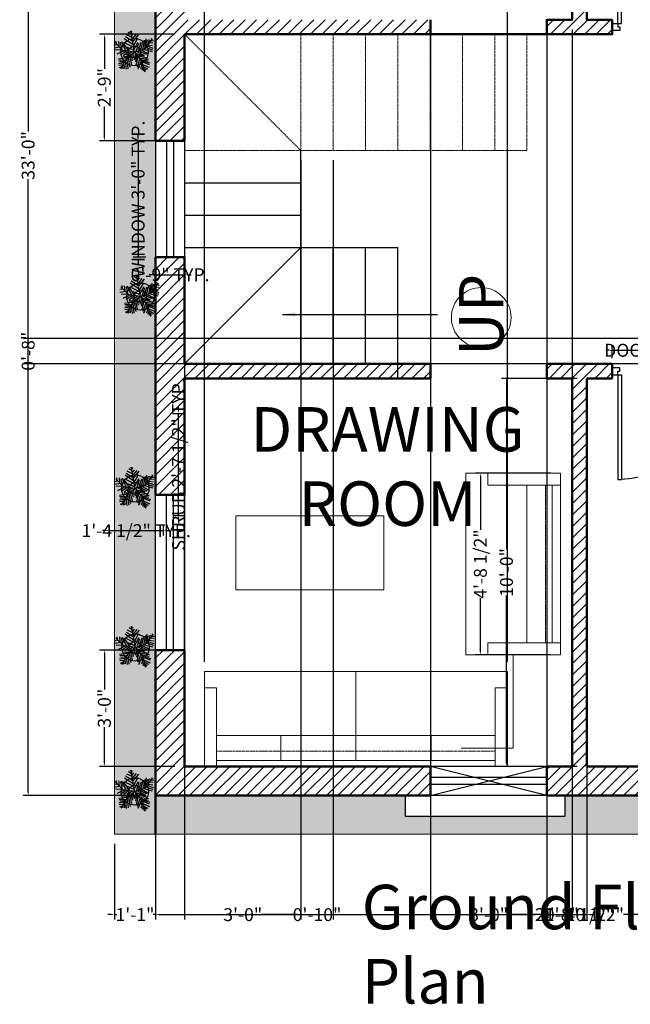
# Model space of a CAD drawing. Units: inches. Extents: x 1265938 to 1266301, y 2357745 to 2358240.
# Tile 1 of 4: x 1265942 to 1266131, y 2357745 to 2358050. Entities that reach past the tile are written whole.
import ezdxf

# ---------------------------------------------------------------- set-up
doc = ezdxf.new("R2010")
doc.units = ezdxf.units.IN
doc.header["$MEASUREMENT"] = 0
doc.linetypes.add('20230926_Unit Plans$0$HIDDEN', pattern=[0.375, 0.25, -0.125])
for name, color, linetype, lineweight in [('A-ANNO-SYMB', 7, 'Continuous', 18), ('A-ANNO-TEXT', 7, 'Continuous', 25), ('A-AREA-IDEN', 7, 'Continuous', 18), ('A-DOOR', 4, 'Continuous', 25), ('A-FLOR-STRS', 7, 'Continuous', 25), ('A-FLOR-STRS-OVHD', 6, '20230926_Unit Plans$0$HIDDEN', 18), ('A-FURN', 8, 'Continuous', 18), ('A-FURN-HIDN', 8, '20230926_Unit Plans$0$HIDDEN', 13), ('A-WALL-PATT', 8, 'Continuous', 13), ('L-PLNT', 3, 'Continuous', 18), ('L-PLNT-BEDS', 3, 'Continuous', 18), ('L-PLNT-PATT', 3, 'Continuous', 13), ('WALL', 7, 'Continuous', 50), ('WINDOW', 2, 'Continuous', 25), ('YQ_DIM', 3, 'Continuous', 18)]:
    doc.layers.add(name, color=color, linetype=linetype, lineweight=lineweight)
doc.layers.add('Layer2', color=102, linetype='Continuous')
doc.layers.add('RAMP SLOPE', color=8, linetype='Continuous')
doc.styles.get("Standard").update_dxf_attribs({"font": 'arial.ttf'})
doc.styles.add('YQ_DIM', font='SUPEROS.SHX', dxfattribs={"width": 0.8, "bigfont": 'HZDX.SHX'})
doc.dimstyles.new('yqi0', dxfattribs={"dimscale": 0, "dimtxt": 4, "dimasz": 1, "dimexe": 1.5, "dimexo": 3, "dimgap": 0.5, "dimtad": 0, "dimdsep": 46, "dimlunit": 4, "dimtxsty": 'Standard', "dimcen": 0, "dimclrd": 256, "dimclre": 256, "dimclrt": 7, "dimadec": 1, "dimazin": 2, "dimtfac": 1, "dimtix": 1, "dimtmove": 2, "dimatfit": 2, "dimfxl": 1, "dimtolj": 1, "dimtzin": 0, "dimarcsym": 0})

# ---------------------------------------------------------------- blocks, each defined once
blk = doc.blocks.new('WD_WIN4')
for p, q in [((-0.5, 0.5), (0.5, 0.5)), ((-0.5, 0.12), (0.5, 0.12)), ((-0.5, -0.12), (0.5, -0.12)), ((-0.5, -0.5), (0.5, -0.5))]:
    blk.add_line(p, q)
blk = doc.blocks.new('DR_D01')
for p, q in [((-0.45, 0.93), (-0.42, 0.93)), ((-0.45, 0.03), (-0.45, 0.93)), ((-0.42, 0.03), (-0.42, 0.93)), ((-0.5, 0.03), (-0.42, 0.03)), ((-0.5, 0.03), (-0.5, -0.03)), ((-0.45, 0.03), (-0.45, 0)), ((-0.45, 0), (-0.435, 0)), ((-0.435, 0), (-0.435, -0.03)), ((0.435, 0), (0.435, -0.03)), ((0.45, 0), (0.435, 0)), ((0.45, 0.03), (0.45, 0)), ((0.5, 0.03), (0.45, 0.03)), ((0.5, -0.03), (0.5, 0.03)), ((-0.435, -0.03), (-0.5, -0.03)), ((0.435, -0.03), (0.5, -0.03))]:
    blk.add_line(p, q)
blk.add_arc((-0.4602, 0.0206), 0.9103, 0.59152, 87.46644)
blk = doc.blocks.new('Trees - Metric')
at = {"layer": 'Layer2'}
for p, q in [((-258.7244, 1362.456), (-332.3336, 1421.4348)), ((0, 0), (-266.7, 1447.8)), ((-231.1146, 1315.2628), (-166.7002, 1421.4348)), ((-1234.059, 536.7274), (-1252.4486, 737.2604)), ((-1105.2302, 725.4494), (-1077.6458, 395.1732)), ((-902.8176, 713.6638), (-617.5756, 100.2538)), ((-93.091, 489.5342), (-700.3796, 902.3858)), ((-129.8956, 713.6638), (-626.7704, 1032.1544)), ((-185.1152, 1008.5578), (-553.1612, 1185.4942)), ((-221.9198, 1197.3052), (-433.5526, 1338.8594)), ((-194.31, 1102.9442), (-65.4812, 1256.284)), ((-148.3106, 914.1968), (118.5418, 1220.9018)), ((-129.8956, 701.8528), (265.7602, 1185.4942)), ((-74.7014, 418.7444), (219.7608, 961.39)), ((-28.6766, 171.0436), (228.9556, 678.2816)), ((412.9786, 147.447), (587.8068, 796.2392)), ((560.197, 182.8292), (698.2206, 819.8358)), ((685.8, 228.6), (1219.2, 914.4)), ((689.0258, 230.0224), (790.2448, 914.1968)), ((808.6344, 784.4282), (827.0494, 418.7444)), ((891.4384, 831.6214), (946.658, 572.1096)), ((983.4626, 867.0036), (1066.2666, 725.4494)), ((1112.2914, 760.8316), (1296.3144, 784.4282)), ((1121.4862, 925.9824), (1149.0706, 831.6214)), ((-1206.4492, 501.3198), (-1418.082, 465.9376)), ((-1031.621, 347.98), (-1399.667, 277.1902)), ((-800.1, 114.3), (-1333.5, 647.7)), ((-847.598, 159.2326), (-1326.0578, 135.636)), ((-718.7946, 88.4682), (-1215.644, -147.447)), ((-976.4268, 666.4706), (-884.4026, 194.6402)), ((-543.9664, 76.6572), (-967.2066, -206.4512)), ((0, 0), (-800.1, 114.3)), ((-369.1382, 53.086), (-783.1836, 642.874)), ((-405.9428, 53.086), (-764.794, -241.8334)), ((-617.5756, 607.4918), (-74.7014, 347.98)), ((0, 0), (-571.5, -495.3)), ((-166.7002, 29.4894), (-543.9664, -206.4512)), ((-525.5514, 347.98), (-28.6766, 123.8504)), ((0, 0), (685.8, 228.6)), ((0, 0), (457.2, -571.5)), ((100.1268, 41.275), (284.1498, 619.2774)), ((164.5412, 41.275), (661.416, -218.2368)), ((256.5654, 88.4682), (449.7832, 666.4706)), ((284.1498, 88.4682), (781.0246, -147.447)), ((458.978, 147.447), (891.4384, -88.4682)), ((615.4166, 194.6402), (1185.8752, 41.275)), ((753.4148, 312.5978), (1222.6798, 159.2326)), ((845.439, 418.7444), (1241.0948, 277.1902)), ((919.0482, 501.3198), (1222.6798, 454.152)), ((1029.462, 654.685), (1241.0948, 631.0884)), ((-442.7474, -383.3876), (-1086.8406, -477.7486)), ((-617.5756, -548.5384), (-1077.6458, -560.324)), ((-681.9646, -666.496), (-1022.4262, -654.685)), ((-571.5, -495.3), (-952.5, -1143)), ((-387.5278, -324.4088), (-764.794, -324.4088)), ((-635.9652, -607.5172), (-580.771, -1150.1374)), ((-525.5514, -465.963), (-451.9422, -1126.5408)), ((-166.7002, -147.447), (-507.1618, -253.619)), ((-433.5526, -383.3876), (-323.1134, -1020.3688)), ((-341.5284, -289.0012), (-221.9198, -831.6214)), ((-240.3094, -218.2368), (-157.5054, -595.7062)), ((-120.7008, -88.4682), (-93.091, -371.5766)), ((63.3222, -76.6826), (-37.8714, -513.1308)), ((44.9326, -64.897), (615.4166, -241.8334)), ((127.7366, -159.258), (54.1274, -654.685)), ((228.9556, -289.0012), (90.932, -914.1968)), ((357.759, -430.5554), (164.5412, -1020.3688)), ((192.151, -230.0224), (817.8292, -371.5766)), ((458.978, -572.1096), (210.5406, -1161.923)), ((311.7596, -383.3876), (937.4378, -477.7486)), ((412.9786, -501.3452), (919.0482, -583.9206)), ((457.2, -571.5), (685.8, -1333.5)), ((468.1982, -572.1096), (1029.462, -737.2604)), ((486.5878, -642.8994), (983.4626, -843.4324)), ((-718.7946, -737.2604), (-1086.8406, -796.2392)), ((-783.1836, -867.029), (-1077.6458, -902.4112)), ((-875.2078, -1008.5832), (-1040.8412, -1079.3476)), ((-829.2084, -937.7934), (-810.7934, -1126.5408)), ((-737.1842, -784.4536), (-709.5744, -1114.7298)), ((514.1976, -772.6426), (403.7838, -1138.3264)), ((578.612, -961.39), (495.7826, -1232.7128)), ((541.8074, -831.6214), (992.6574, -1032.1544)), ((578.612, -973.1756), (873.0488, -1138.3264)), ((624.6114, -1161.923), (587.8068, -1291.6916)), ((624.6114, -1102.9442), (781.0246, -1209.1162)), ((679.8056, -1268.095), (716.6102, -1291.6916))]:
    blk.add_line(p, q, dxfattribs=at)
blk = doc.blocks.new('A$Cbdbf8f2b')
at = {"layer": 'RAMP SLOPE'}
for radius in [7.17, 3.22]:
    blk.add_circle((13.77, 14.11), radius, dxfattribs=at)
at = {"xscale": 0.0077264756515533, "yscale": 0.0077264756515533, "zscale": 0.0077264756515533}
blk.add_blockref('Trees - Metric', (13.77, 14.11), dxfattribs=at)
blk = doc.blocks.new('*D16')
at = {"layer": 'Defpoints', "color": 0, "transparency": 16777216}
for p in [(1265986.27, 2357927.89), (1265991, 2357927.89), (1265986.27, 2357896.34)]:
    blk.add_point(p, dxfattribs=at)
at = {"layer": 'YQ_DIM', "lineweight": -2, "transparency": 16777216}
for p, q in [((1265991, 2357928.89), (1265991, 2357929.89)), ((1265989.27, 2357927.89), (1265992.5, 2357927.89)), ((1265991, 2357896.34), (1265991, 2357927.89)), ((1265989.27, 2357896.34), (1265992.5, 2357896.34)), ((1265991, 2357895.34), (1265991, 2357894.34))]:
    blk.add_line(p, q, dxfattribs=at)
at = {"layer": 'YQ_DIM', "transparency": 16777216}
for points in [[(1265990.83, 2357928.89), (1265991.16, 2357928.89), (1265991, 2357927.89)], [(1265990.83, 2357895.34), (1265991.16, 2357895.34), (1265991, 2357896.34)]]:
    blk.add_solid(points, dxfattribs=at)
at = {"layer": 'YQ_DIM', "color": 7, "transparency": 16777216, "insert": (1265991, 2357912.11), "char_height": 4, "attachment_point": 5, "rotation": 90}
blk.add_mtext('\\A1;SHRUB 2\'-7 1/2" TYP.', dxfattribs=at)
blk = doc.blocks.new('*D17')
at = {"layer": 'Defpoints', "color": 0, "transparency": 16777216}
for p in [(1265969.52, 2357896.34), (1265986.27, 2357896.34), (1265986.27, 2357891.61)]:
    blk.add_point(p, dxfattribs=at)
at = {"layer": 'YQ_DIM', "lineweight": -2, "transparency": 16777216}
for p, q in [((1265969.52, 2357893.34), (1265969.52, 2357890.11)), ((1265986.27, 2357893.34), (1265986.27, 2357890.11)), ((1265968.52, 2357891.61), (1265967.52, 2357891.61)), ((1265969.52, 2357891.61), (1265986.27, 2357891.61)), ((1265987.27, 2357891.61), (1265988.27, 2357891.61))]:
    blk.add_line(p, q, dxfattribs=at)
at = {"layer": 'YQ_DIM', "transparency": 16777216}
for points in [[(1265968.52, 2357891.78), (1265968.52, 2357891.44), (1265969.52, 2357891.61)], [(1265987.27, 2357891.78), (1265987.27, 2357891.44), (1265986.27, 2357891.61)]]:
    blk.add_solid(points, dxfattribs=at)
at = {"layer": 'YQ_DIM', "color": 7, "transparency": 16777216, "insert": (1265977.89, 2357891.61), "char_height": 4, "attachment_point": 5}
blk.add_mtext('\\A1;1\'-4 1/2" TYP.', dxfattribs=at)
blk = doc.blocks.new('*D22')
at = {"layer": 'Defpoints', "color": 0, "transparency": 16777216}
for p in [(1265983.89, 2358012.18), (1265978.49, 2357976.18), (1265983.89, 2357976.18)]:
    blk.add_point(p, dxfattribs=at)
at = {"layer": 'YQ_DIM', "lineweight": -2, "transparency": 16777216}
for p, q in [((1265978.49, 2358013.18), (1265978.49, 2358014.18)), ((1265980.89, 2358012.18), (1265976.99, 2358012.18)), ((1265978.49, 2358012.18), (1265978.49, 2357976.18)), ((1265980.89, 2357976.18), (1265976.99, 2357976.18)), ((1265978.49, 2357975.18), (1265978.49, 2357974.18))]:
    blk.add_line(p, q, dxfattribs=at)
at = {"layer": 'YQ_DIM', "transparency": 16777216}
for points in [[(1265978.32, 2358013.18), (1265978.66, 2358013.18), (1265978.49, 2358012.18)], [(1265978.32, 2357975.18), (1265978.66, 2357975.18), (1265978.49, 2357976.18)]]:
    blk.add_solid(points, dxfattribs=at)
at = {"layer": 'YQ_DIM', "color": 7, "transparency": 16777216, "insert": (1265978.49, 2357994.18), "char_height": 4, "attachment_point": 5, "rotation": 90}
blk.add_mtext('\\A1;WINDOW 3\'-0" TYP.', dxfattribs=at)
blk = doc.blocks.new('*D23')
at = {"layer": 'Defpoints', "color": 0, "transparency": 16777216}
for p in [(1265983.89, 2357976.18), (1265992.89, 2357976.18), (1265992.89, 2357970.78)]:
    blk.add_point(p, dxfattribs=at)
at = {"layer": 'YQ_DIM', "lineweight": -2, "transparency": 16777216}
for p, q in [((1265983.89, 2357973.18), (1265983.89, 2357969.28)), ((1265992.89, 2357973.18), (1265992.89, 2357969.28)), ((1265982.89, 2357970.78), (1265981.89, 2357970.78)), ((1265983.89, 2357970.78), (1265992.89, 2357970.78)), ((1265993.89, 2357970.78), (1265994.89, 2357970.78))]:
    blk.add_line(p, q, dxfattribs=at)
at = {"layer": 'YQ_DIM', "transparency": 16777216}
for points in [[(1265982.89, 2357970.95), (1265982.89, 2357970.61), (1265983.89, 2357970.78)], [(1265993.89, 2357970.95), (1265993.89, 2357970.61), (1265992.89, 2357970.78)]]:
    blk.add_solid(points, dxfattribs=at)
at = {"layer": 'YQ_DIM', "color": 7, "transparency": 16777216, "insert": (1265988.39, 2357970.78), "char_height": 4, "attachment_point": 5}
blk.add_mtext('\\A1;0\'-9" TYP.', dxfattribs=at)
blk = doc.blocks.new('*D26')
at = {"layer": 'Defpoints', "color": 0, "transparency": 16777216}
for p in [(1266161.26, 2357947.41), (1266125.26, 2357942.01), (1266161.26, 2357942.01)]:
    blk.add_point(p, dxfattribs=at)
at = {"layer": 'YQ_DIM', "lineweight": -2, "transparency": 16777216}
for p, q in [((1266124.26, 2357947.41), (1266123.26, 2357947.41)), ((1266125.26, 2357945.01), (1266125.26, 2357948.91)), ((1266125.26, 2357947.41), (1266161.26, 2357947.41)), ((1266161.26, 2357945.01), (1266161.26, 2357948.91)), ((1266162.26, 2357947.41), (1266163.26, 2357947.41))]:
    blk.add_line(p, q, dxfattribs=at)
at = {"layer": 'YQ_DIM', "transparency": 16777216}
for points in [[(1266124.26, 2357947.58), (1266124.26, 2357947.24), (1266125.26, 2357947.41)], [(1266162.26, 2357947.58), (1266162.26, 2357947.24), (1266161.26, 2357947.41)]]:
    blk.add_solid(points, dxfattribs=at)
at = {"layer": 'YQ_DIM', "color": 7, "transparency": 16777216, "insert": (1266143.26, 2357947.41), "char_height": 4, "attachment_point": 5}
blk.add_mtext('\\A1;DOOR 3\'-0" TYP.', dxfattribs=at)
blk = doc.blocks.new('*D36')
at = {"layer": 'Defpoints', "color": 0, "transparency": 16777216}
for p in [(1265983.89, 2357809.68), (1266246.39, 2357809.68), (1266246.39, 2357772.83)]:
    blk.add_point(p, dxfattribs=at)
at = {"layer": 'YQ_DIM', "lineweight": -2, "transparency": 16777216}
for p, q in [((1265983.89, 2357806.68), (1265983.89, 2357771.33)), ((1266246.39, 2357806.68), (1266246.39, 2357771.33)), ((1265984.89, 2357772.83), (1266101.52, 2357772.83)), ((1266245.39, 2357772.83), (1266128.76, 2357772.83))]:
    blk.add_line(p, q, dxfattribs=at)
at = {"layer": 'YQ_DIM', "transparency": 16777216}
for points in [[(1265984.89, 2357773), (1265984.89, 2357772.66), (1265983.89, 2357772.83)], [(1266245.39, 2357773), (1266245.39, 2357772.66), (1266246.39, 2357772.83)]]:
    blk.add_solid(points, dxfattribs=at)
at = {"layer": 'YQ_DIM', "color": 7, "transparency": 16777216, "insert": (1266115.14, 2357772.83), "char_height": 4, "attachment_point": 5}
blk.add_mtext('\\A1;21\'-10 1/2"', dxfattribs=at)
blk = doc.blocks.new('*D37')
at = {"layer": 'Defpoints', "color": 0, "transparency": 16777216}
for p in [(1265944.45, 2358205.68), (1265983.89, 2358205.68), (1265983.89, 2357809.68)]:
    blk.add_point(p, dxfattribs=at)
at = {"layer": 'YQ_DIM', "lineweight": -2, "transparency": 16777216}
for p, q in [((1265980.89, 2358205.68), (1265942.95, 2358205.68)), ((1265944.45, 2358204.68), (1265944.45, 2358015.05)), ((1265944.45, 2357810.68), (1265944.45, 2358000.31)), ((1265980.89, 2357809.68), (1265942.95, 2357809.68))]:
    blk.add_line(p, q, dxfattribs=at)
at = {"layer": 'YQ_DIM', "transparency": 16777216}
for points in [[(1265944.29, 2358204.68), (1265944.62, 2358204.68), (1265944.45, 2358205.68)], [(1265944.29, 2357810.68), (1265944.62, 2357810.68), (1265944.45, 2357809.68)]]:
    blk.add_solid(points, dxfattribs=at)
at = {"layer": 'YQ_DIM', "color": 7, "transparency": 16777216, "insert": (1265944.45, 2358007.68), "char_height": 4, "attachment_point": 5, "rotation": 90}
blk.add_mtext('\\A1;33\'-0"', dxfattribs=at)
blk = doc.blocks.new('*D42')
at = {"layer": 'Defpoints', "color": 0, "transparency": 16777216}
for p in [(1266092.54, 2357938.68), (1266117.39, 2357938.68), (1266117.39, 2357818.68)]:
    blk.add_point(p, dxfattribs=at)
at = {"layer": 'YQ_DIM', "lineweight": -2, "transparency": 16777216}
for p, q in [((1266114.39, 2357938.68), (1266091.04, 2357938.68)), ((1266092.54, 2357937.68), (1266092.54, 2357885.86)), ((1266092.54, 2357819.68), (1266092.54, 2357871.5)), ((1266114.39, 2357818.68), (1266091.04, 2357818.68))]:
    blk.add_line(p, q, dxfattribs=at)
at = {"layer": 'YQ_DIM', "transparency": 16777216}
for points in [[(1266092.37, 2357937.68), (1266092.71, 2357937.68), (1266092.54, 2357938.68)], [(1266092.37, 2357819.68), (1266092.71, 2357819.68), (1266092.54, 2357818.68)]]:
    blk.add_solid(points, dxfattribs=at)
at = {"layer": 'YQ_DIM', "color": 7, "transparency": 16777216, "insert": (1266092.54, 2357878.68), "char_height": 4, "attachment_point": 5, "rotation": 90}
blk.add_mtext('\\A1;10\'-0"', dxfattribs=at)
blk = doc.blocks.new('*D43')
at = {"layer": 'Defpoints', "color": 0, "transparency": 16777216}
for p in [(1265968.04, 2357854.68), (1265992.89, 2357854.68), (1265992.89, 2357818.68)]:
    blk.add_point(p, dxfattribs=at)
at = {"layer": 'YQ_DIM', "lineweight": -2, "transparency": 16777216}
for p, q in [((1265989.89, 2357854.68), (1265966.54, 2357854.68)), ((1265968.04, 2357853.68), (1265968.04, 2357842.5)), ((1265968.04, 2357819.68), (1265968.04, 2357830.87)), ((1265989.89, 2357818.68), (1265966.54, 2357818.68))]:
    blk.add_line(p, q, dxfattribs=at)
at = {"layer": 'YQ_DIM', "transparency": 16777216}
for points in [[(1265967.87, 2357853.68), (1265968.21, 2357853.68), (1265968.04, 2357854.68)], [(1265967.87, 2357819.68), (1265968.21, 2357819.68), (1265968.04, 2357818.68)]]:
    blk.add_solid(points, dxfattribs=at)
at = {"layer": 'YQ_DIM', "color": 7, "transparency": 16777216, "insert": (1265968.04, 2357836.68), "char_height": 4, "attachment_point": 5, "rotation": 90}
blk.add_mtext('\\A1;3\'-0"', dxfattribs=at)
blk = doc.blocks.new('*D44')
at = {"layer": 'Defpoints', "color": 0, "transparency": 16777216}
for p in [(1265968.04, 2358045.18), (1265992.89, 2358045.18), (1265992.89, 2358012.18)]:
    blk.add_point(p, dxfattribs=at)
at = {"layer": 'YQ_DIM', "lineweight": -2, "transparency": 16777216}
for p, q in [((1265989.89, 2358045.18), (1265966.54, 2358045.18)), ((1265968.04, 2358044.18), (1265968.04, 2358034.53)), ((1265968.04, 2358013.18), (1265968.04, 2358022.83)), ((1265989.89, 2358012.18), (1265966.54, 2358012.18))]:
    blk.add_line(p, q, dxfattribs=at)
at = {"layer": 'YQ_DIM', "transparency": 16777216}
for points in [[(1265967.87, 2358044.18), (1265968.21, 2358044.18), (1265968.04, 2358045.18)], [(1265967.87, 2358013.18), (1265968.21, 2358013.18), (1265968.04, 2358012.18)]]:
    blk.add_solid(points, dxfattribs=at)
at = {"layer": 'YQ_DIM', "color": 7, "transparency": 16777216, "insert": (1265968.04, 2358028.68), "char_height": 4, "attachment_point": 5, "rotation": 90}
blk.add_mtext('\\A1;2\'-9"', dxfattribs=at)
blk = doc.blocks.new('*D48')
at = {"layer": 'Defpoints', "color": 0, "transparency": 16777216}
for p in [(1266105.02, 2357818.68), (1266112.89, 2357818.68), (1266112.89, 2357772.83)]:
    blk.add_point(p, dxfattribs=at)
at = {"layer": 'YQ_DIM', "lineweight": -2, "transparency": 16777216}
for p, q in [((1266105.02, 2357815.68), (1266105.02, 2357771.33)), ((1266112.89, 2357815.68), (1266112.89, 2357771.33)), ((1266104.02, 2357772.83), (1266103.02, 2357772.83)), ((1266105.02, 2357772.83), (1266112.89, 2357772.83)), ((1266113.89, 2357772.83), (1266114.89, 2357772.83))]:
    blk.add_line(p, q, dxfattribs=at)
at = {"layer": 'YQ_DIM', "transparency": 16777216}
for points in [[(1266104.02, 2357773), (1266104.02, 2357772.66), (1266105.02, 2357772.83)], [(1266113.89, 2357773), (1266113.89, 2357772.66), (1266112.89, 2357772.83)]]:
    blk.add_solid(points, dxfattribs=at)
at = {"layer": 'YQ_DIM', "color": 7, "transparency": 16777216, "insert": (1266108.96, 2357772.83), "char_height": 4, "attachment_point": 5}
blk.add_mtext('\\A1;0\'-8"', dxfattribs=at)
blk = doc.blocks.new('*D49')
at = {"layer": 'Defpoints', "color": 0, "transparency": 16777216}
for p in [(1266125.26, 2358237.77), (1266117.39, 2358049.68), (1266125.26, 2358049.68)]:
    blk.add_point(p, dxfattribs=at)
at = {"layer": 'YQ_DIM', "lineweight": -2, "transparency": 16777216}
for p, q in [((1266117.39, 2358052.68), (1266117.39, 2358239.27)), ((1266125.26, 2358052.68), (1266125.26, 2358239.27)), ((1266116.39, 2358237.77), (1266115.39, 2358237.77)), ((1266117.39, 2358237.77), (1266125.26, 2358237.77)), ((1266126.26, 2358237.77), (1266127.26, 2358237.77))]:
    blk.add_line(p, q, dxfattribs=at)
at = {"layer": 'YQ_DIM', "transparency": 16777216}
for points in [[(1266116.39, 2358237.93), (1266116.39, 2358237.6), (1266117.39, 2358237.77)], [(1266126.26, 2358237.93), (1266126.26, 2358237.6), (1266125.26, 2358237.77)]]:
    blk.add_solid(points, dxfattribs=at)
at = {"layer": 'YQ_DIM', "color": 7, "transparency": 16777216, "insert": (1266121.33, 2358237.77), "char_height": 4, "attachment_point": 5}
blk.add_mtext('\\A1;0\'-8"', dxfattribs=at)
blk = doc.blocks.new('*D50')
at = {"layer": 'Defpoints', "color": 0, "transparency": 16777216}
for p in [(1265944.45, 2357951.05), (1266183.39, 2357951.05), (1266183.39, 2357943.18)]:
    blk.add_point(p, dxfattribs=at)
at = {"layer": 'YQ_DIM', "lineweight": -2, "transparency": 16777216}
for p, q in [((1265944.45, 2357952.05), (1265944.45, 2357953.05)), ((1266180.39, 2357951.05), (1265942.95, 2357951.05)), ((1265944.45, 2357943.18), (1265944.45, 2357951.05)), ((1266180.39, 2357943.18), (1265942.95, 2357943.18)), ((1265944.45, 2357942.18), (1265944.45, 2357941.18))]:
    blk.add_line(p, q, dxfattribs=at)
at = {"layer": 'YQ_DIM', "transparency": 16777216}
for points in [[(1265944.29, 2357952.05), (1265944.62, 2357952.05), (1265944.45, 2357951.05)], [(1265944.29, 2357942.18), (1265944.62, 2357942.18), (1265944.45, 2357943.18)]]:
    blk.add_solid(points, dxfattribs=at)
at = {"layer": 'YQ_DIM', "color": 7, "transparency": 16777216, "insert": (1265944.45, 2357947.12), "char_height": 4, "attachment_point": 5, "rotation": 90}
blk.add_mtext('\\A1;0\'-8"', dxfattribs=at)
blk = doc.blocks.new('*D51')
at = {"layer": 'Defpoints', "color": 0, "transparency": 16777216}
for p in [(1265992.89, 2358045.18), (1266028.89, 2358009.18), (1266028.89, 2357772.83)]:
    blk.add_point(p, dxfattribs=at)
at = {"layer": 'YQ_DIM', "lineweight": -2, "transparency": 16777216}
for p, q in [((1265992.89, 2358042.18), (1265992.89, 2357771.33)), ((1266028.89, 2358006.18), (1266028.89, 2357771.33)), ((1265993.89, 2357772.83), (1266005.08, 2357772.83)), ((1266027.89, 2357772.83), (1266016.71, 2357772.83))]:
    blk.add_line(p, q, dxfattribs=at)
at = {"layer": 'YQ_DIM', "transparency": 16777216}
for points in [[(1265993.89, 2357773), (1265993.89, 2357772.66), (1265992.89, 2357772.83)], [(1266027.89, 2357773), (1266027.89, 2357772.66), (1266028.89, 2357772.83)]]:
    blk.add_solid(points, dxfattribs=at)
at = {"layer": 'YQ_DIM', "color": 7, "transparency": 16777216, "insert": (1266010.89, 2357772.83), "char_height": 4, "attachment_point": 5}
blk.add_mtext('\\A1;3\'-0"', dxfattribs=at)
blk = doc.blocks.new('*D52')
at = {"layer": 'Defpoints', "color": 0, "transparency": 16777216}
for p in [(1266028.89, 2358009.18), (1266038.89, 2358009.18), (1266038.89, 2357772.83)]:
    blk.add_point(p, dxfattribs=at)
at = {"layer": 'YQ_DIM', "lineweight": -2, "transparency": 16777216}
for p, q in [((1266028.89, 2358006.18), (1266028.89, 2357771.33)), ((1266038.89, 2358006.18), (1266038.89, 2357771.33)), ((1266027.89, 2357772.83), (1266026.89, 2357772.83)), ((1266028.89, 2357772.83), (1266038.89, 2357772.83)), ((1266039.89, 2357772.83), (1266040.89, 2357772.83))]:
    blk.add_line(p, q, dxfattribs=at)
at = {"layer": 'YQ_DIM', "transparency": 16777216}
for points in [[(1266027.89, 2357773), (1266027.89, 2357772.66), (1266028.89, 2357772.83)], [(1266039.89, 2357773), (1266039.89, 2357772.66), (1266038.89, 2357772.83)]]:
    blk.add_solid(points, dxfattribs=at)
at = {"layer": 'YQ_DIM', "color": 7, "transparency": 16777216, "insert": (1266033.89, 2357772.83), "char_height": 4, "attachment_point": 5}
blk.add_mtext('\\A1;0\'-10"', dxfattribs=at)
blk = doc.blocks.new('*D53')
at = {"layer": 'Defpoints', "color": 0, "transparency": 16777216}
for p in [(1266069.02, 2358049.68), (1266105.02, 2358049.68), (1266105.02, 2357772.83)]:
    blk.add_point(p, dxfattribs=at)
at = {"layer": 'YQ_DIM', "lineweight": -2, "transparency": 16777216}
for p, q in [((1266069.02, 2358046.68), (1266069.02, 2357771.33)), ((1266105.02, 2358046.68), (1266105.02, 2357771.33)), ((1266070.02, 2357772.83), (1266081.2, 2357772.83)), ((1266104.02, 2357772.83), (1266092.83, 2357772.83))]:
    blk.add_line(p, q, dxfattribs=at)
at = {"layer": 'YQ_DIM', "transparency": 16777216}
for points in [[(1266070.02, 2357773), (1266070.02, 2357772.66), (1266069.02, 2357772.83)], [(1266104.02, 2357773), (1266104.02, 2357772.66), (1266105.02, 2357772.83)]]:
    blk.add_solid(points, dxfattribs=at)
at = {"layer": 'YQ_DIM', "color": 7, "transparency": 16777216, "insert": (1266087.02, 2357772.83), "char_height": 4, "attachment_point": 5}
blk.add_mtext('\\A1;3\'-0"', dxfattribs=at)
blk = doc.blocks.new('*D54')
at = {"layer": 'Defpoints', "color": 0, "transparency": 16777216}
for p in [(1266105.02, 2358049.68), (1266112.89, 2358049.68), (1266112.89, 2357772.83)]:
    blk.add_point(p, dxfattribs=at)
at = {"layer": 'YQ_DIM', "lineweight": -2, "transparency": 16777216}
for p, q in [((1266105.02, 2358046.68), (1266105.02, 2357771.33)), ((1266112.89, 2358046.68), (1266112.89, 2357771.33)), ((1266104.02, 2357772.83), (1266103.02, 2357772.83)), ((1266105.02, 2357772.83), (1266112.89, 2357772.83)), ((1266113.89, 2357772.83), (1266114.89, 2357772.83))]:
    blk.add_line(p, q, dxfattribs=at)
at = {"layer": 'YQ_DIM', "transparency": 16777216}
for points in [[(1266104.02, 2357773), (1266104.02, 2357772.66), (1266105.02, 2357772.83)], [(1266113.89, 2357773), (1266113.89, 2357772.66), (1266112.89, 2357772.83)]]:
    blk.add_solid(points, dxfattribs=at)
at = {"layer": 'YQ_DIM', "color": 7, "transparency": 16777216, "insert": (1266108.95, 2357772.83), "char_height": 4, "attachment_point": 5}
blk.add_mtext('\\A1;0\'-8"', dxfattribs=at)
blk = doc.blocks.new('*D55')
at = {"layer": 'Defpoints', "color": 0, "transparency": 16777216}
for p in [(1266092.81, 2358237.77), (1265999.06, 2357848.06), (1266092.81, 2357848.06)]:
    blk.add_point(p, dxfattribs=at)
at = {"layer": 'YQ_DIM', "lineweight": -2, "transparency": 16777216}
for p, q in [((1265999.06, 2357851.06), (1265999.06, 2358239.27)), ((1266092.81, 2357851.06), (1266092.81, 2358239.27)), ((1266000.06, 2358237.77), (1266038.58, 2358237.77)), ((1266091.81, 2358237.77), (1266053.28, 2358237.77))]:
    blk.add_line(p, q, dxfattribs=at)
at = {"layer": 'YQ_DIM', "transparency": 16777216}
for points in [[(1266000.06, 2358237.93), (1266000.06, 2358237.6), (1265999.06, 2358237.77)], [(1266091.81, 2358237.93), (1266091.81, 2358237.6), (1266092.81, 2358237.77)]]:
    blk.add_solid(points, dxfattribs=at)
at = {"layer": 'YQ_DIM', "color": 7, "transparency": 16777216, "insert": (1266045.93, 2358237.77), "char_height": 4, "attachment_point": 5}
blk.add_mtext('\\A1;7\'-10"', dxfattribs=at)
blk = doc.blocks.new('*D56')
at = {"layer": 'Defpoints', "color": 0, "transparency": 16777216}
for p in [(1266084.45, 2357909.42), (1266109.3, 2357909.42), (1266109.3, 2357853.17)]:
    blk.add_point(p, dxfattribs=at)
at = {"layer": 'YQ_DIM', "lineweight": -2, "transparency": 16777216}
for p, q in [((1266106.3, 2357909.42), (1266082.95, 2357909.42)), ((1266084.45, 2357908.42), (1266084.45, 2357891.85)), ((1266084.45, 2357854.17), (1266084.45, 2357870.73)), ((1266106.3, 2357853.17), (1266082.95, 2357853.17))]:
    blk.add_line(p, q, dxfattribs=at)
at = {"layer": 'YQ_DIM', "transparency": 16777216}
for points in [[(1266084.29, 2357908.42), (1266084.62, 2357908.42), (1266084.45, 2357909.42)], [(1266084.29, 2357854.17), (1266084.62, 2357854.17), (1266084.45, 2357853.17)]]:
    blk.add_solid(points, dxfattribs=at)
at = {"layer": 'YQ_DIM', "color": 7, "transparency": 16777216, "insert": (1266084.45, 2357881.29), "char_height": 4, "attachment_point": 5, "rotation": 90}
blk.add_mtext('\\A1;4\'-8 1/2"', dxfattribs=at)
blk = doc.blocks.new('*D57')
at = {"layer": 'Defpoints', "color": 0, "transparency": 16777216}
for p in [(1265971.14, 2357797.68), (1265983.89, 2357797.68), (1265983.89, 2357772.83)]:
    blk.add_point(p, dxfattribs=at)
at = {"layer": 'YQ_DIM', "lineweight": -2, "transparency": 16777216}
for p, q in [((1265971.14, 2357794.68), (1265971.14, 2357771.33)), ((1265983.89, 2357794.68), (1265983.89, 2357771.33)), ((1265970.14, 2357772.83), (1265969.14, 2357772.83)), ((1265971.14, 2357772.83), (1265971.89, 2357772.83)), ((1265983.89, 2357772.83), (1265983.14, 2357772.83)), ((1265984.89, 2357772.83), (1265985.89, 2357772.83))]:
    blk.add_line(p, q, dxfattribs=at)
at = {"layer": 'YQ_DIM', "transparency": 16777216}
for points in [[(1265970.14, 2357773), (1265970.14, 2357772.66), (1265971.14, 2357772.83)], [(1265984.89, 2357773), (1265984.89, 2357772.66), (1265983.89, 2357772.83)]]:
    blk.add_solid(points, dxfattribs=at)
at = {"layer": 'YQ_DIM', "color": 7, "transparency": 16777216, "insert": (1265977.52, 2357772.83), "char_height": 4, "attachment_point": 5}
blk.add_mtext('\\A1;1\'-1"', dxfattribs=at)
blk = doc.blocks.new('*D59')
at = {"layer": 'Defpoints', "color": 0, "transparency": 16777216}
for p in [(1266112.89, 2357938.68), (1266117.39, 2357938.68), (1266117.39, 2357772.83)]:
    blk.add_point(p, dxfattribs=at)
at = {"layer": 'YQ_DIM', "lineweight": -2, "transparency": 16777216}
for p, q in [((1266112.89, 2357935.68), (1266112.89, 2357771.33)), ((1266117.39, 2357935.68), (1266117.39, 2357771.33)), ((1266111.89, 2357772.83), (1266110.89, 2357772.83)), ((1266112.89, 2357772.83), (1266117.39, 2357772.83)), ((1266118.39, 2357772.83), (1266119.39, 2357772.83))]:
    blk.add_line(p, q, dxfattribs=at)
at = {"layer": 'YQ_DIM', "transparency": 16777216}
for points in [[(1266111.89, 2357773), (1266111.89, 2357772.66), (1266112.89, 2357772.83)], [(1266118.39, 2357773), (1266118.39, 2357772.66), (1266117.39, 2357772.83)]]:
    blk.add_solid(points, dxfattribs=at)
at = {"layer": 'YQ_DIM', "color": 7, "transparency": 16777216, "insert": (1266115.14, 2357772.83), "char_height": 4, "attachment_point": 5}
blk.add_mtext('\\A1;0\'-4 1/2"', dxfattribs=at)

msp = doc.modelspace()

# ---------------------------------------------------------------- hatches: boundary and pattern name
at = {"layer": 'A-WALL-PATT'}
h = msp.add_hatch(dxfattribs=at)
h.set_pattern_fill('ANSI31', color=256, scale=20)
h.paths.add_polyline_path([(1266117.39, 2358196.681), (1266112.89, 2358196.681), (1266112.89, 2358049.681), (1266105.016, 2358049.681), (1266105.016, 2358045.181), (1266125.264, 2358045.181), (1266125.264, 2358049.681), (1266117.39, 2358049.681)])
h = msp.add_hatch(dxfattribs=at)
h.set_pattern_fill('ANSI31', color=256, scale=20)
h.paths.add_polyline_path([(1266069.016, 2358049.681), (1265992.89, 2358049.681), (1265992.89, 2358099.181), (1265983.89, 2358099.181), (1265983.89, 2358012.181), (1265992.89, 2358012.181), (1265992.89, 2358045.181), (1266069.016, 2358045.181)])
h.paths.add_polyline_path([(1266246.39, 2358049.681), (1266246.39, 2358099.181), (1266237.39, 2358099.181), (1266237.39, 2358049.681), (1266161.264, 2358049.681), (1266161.264, 2358045.181), (1266178.89, 2358045.181), (1266178.89, 2357987.055), (1266183.39, 2357987.055), (1266183.39, 2358045.181), (1266237.39, 2358045.181), (1266237.39, 2358029.655), (1266246.39, 2358029.655)])
h.paths.add_polyline_path([(1265992.89, 2357938.681), (1266058.89, 2357938.681), (1266058.89, 2357943.181), (1265992.89, 2357943.181), (1265992.89, 2357976.181), (1265983.89, 2357976.181), (1265983.89, 2357967.701), (1265984.307, 2357966.989), (1265983.89, 2357967.035), (1265983.89, 2357902.681), (1265992.89, 2357902.681)])
h.paths.add_polyline_path([(1266069.016, 2357943.181), (1266058.89, 2357943.181), (1266058.89, 2357938.681), (1266069.016, 2357938.681)])
h.paths.add_polyline_path([(1266125.264, 2357943.181), (1266105.016, 2357943.181), (1266105.016, 2357938.681), (1266112.89, 2357938.681), (1266112.89, 2357818.681), (1266105.024, 2357818.681), (1266105.024, 2357809.681), (1266112.898, 2357809.681), (1266153.39, 2357809.681), (1266153.39, 2357818.681), (1266117.39, 2357818.681), (1266117.39, 2357938.681), (1266125.264, 2357938.681)])
h.paths.add_polyline_path([(1266069.024, 2357818.681), (1265999.055, 2357818.681), (1265992.89, 2357818.681), (1265992.89, 2357854.681), (1265983.89, 2357854.681), (1265983.89, 2357809.681), (1266069.024, 2357809.681)])
h.paths.add_polyline_path([(1266246.39, 2358005.655), (1266237.39, 2358005.655), (1266237.39, 2357943.181), (1266161.264, 2357943.181), (1266161.264, 2357938.681), (1266237.39, 2357938.681), (1266237.39, 2357818.681), (1266201.39, 2357818.681), (1266201.39, 2357809.681), (1266246.39, 2357809.681)])
at = {"layer": 'L-PLNT-PATT'}
h = msp.add_hatch(dxfattribs=at)
h.set_pattern_fill('GRASS', color=256, scale=4)
h.paths.add_polyline_path([(1265983.89, 2358205.681), (1265971.14, 2358205.681), (1265971.14, 2357797.681), (1265983.89, 2357797.681)])
h = msp.add_hatch(dxfattribs=at)
h.set_pattern_fill('GRASS', color=256, scale=4)
h.paths.add_polyline_path([(1266246.39, 2357809.681), (1266201.39, 2357809.681), (1266153.39, 2357809.681), (1266112.89, 2357809.681), (1266110.75, 2357809.681), (1266110.75, 2357803.243), (1266061.166, 2357803.243), (1266061.166, 2357809.681), (1265983.89, 2357809.681), (1265983.89, 2357797.681), (1266246.39, 2357797.681)])

# ---------------------------------------------------------------- linework, layer by layer
at = {"layer": 'A-ANNO-SYMB'}
msp.add_circle((1266084.716, 2357957.548), 9.238, dxfattribs=at)
at = {"layer": 'A-DOOR'}
for p, q in [((1266069.024, 2357809.681), (1266105.024, 2357818.681)), ((1266105.024, 2357809.681), (1266069.024, 2357818.681)), ((1266105.024, 2357818.681), (1266105.024, 2357809.681))]:
    msp.add_line(p, q, dxfattribs=at)
at = {"layer": 'A-FLOR-STRS'}
for p, q in [((1266028.89, 2357943.181), (1266028.89, 2358009.181)), ((1265992.89, 2357999.181), (1266028.89, 2357999.181)), ((1265992.89, 2357989.181), (1266028.89, 2357989.181)), ((1265992.89, 2357979.181), (1266058.89, 2357979.181)), ((1266028.89, 2357979.181), (1265992.89, 2357943.181)), ((1266038.89, 2357943.181), (1266038.89, 2357979.181)), ((1266048.89, 2357943.181), (1266048.89, 2357979.181)), ((1266058.89, 2357938.681), (1266058.89, 2357979.181)), ((1266028.89, 2357943.181), (1266028.89, 2357976.181)), ((1266061.166, 2357809.681), (1266061.166, 2357803.243)), ((1266110.75, 2357803.243), (1266110.75, 2357809.681)), ((1266061.166, 2357803.243), (1266110.75, 2357803.243))]:
    msp.add_line(p, q, dxfattribs=at)
at = {"layer": 'A-FLOR-STRS-OVHD'}
for p, q in [((1266028.89, 2358009.181), (1265992.89, 2358045.181)), ((1266028.89, 2358009.181), (1266028.89, 2358045.181)), ((1266038.89, 2358009.181), (1266038.89, 2358045.181)), ((1266048.89, 2358009.181), (1266048.89, 2358045.181)), ((1266058.89, 2358009.181), (1266058.89, 2358045.181)), ((1266068.89, 2358009.181), (1266068.89, 2358045.181)), ((1266078.89, 2358009.181), (1266078.89, 2358045.181)), ((1266088.89, 2358009.181), (1266088.89, 2358045.181)), ((1266098.89, 2358009.181), (1266098.89, 2358045.181)), ((1265992.89, 2358009.181), (1266098.89, 2358009.181))]:
    msp.add_line(p, q, dxfattribs=at)
at = {"layer": 'A-FURN'}
for p, q in [((1266086.742, 2357905.666), (1266086.742, 2357909.416)), ((1266086.742, 2357905.666), (1266109.304, 2357905.666)), ((1266098.844, 2357856.916), (1266098.844, 2357905.666)), ((1266106.704, 2357856.916), (1266106.704, 2357905.666)), ((1266086.742, 2357856.916), (1266109.304, 2357856.916)), ((1266086.742, 2357856.916), (1266086.742, 2357853.166)), ((1266045.93, 2357828.208), (1266045.93, 2357848.056)), ((1265999.055, 2357843.016), (1266002.805, 2357843.016)), ((1266002.805, 2357843.016), (1266002.805, 2357818.681)), ((1266092.805, 2357843.016), (1266089.055, 2357843.016)), ((1266089.055, 2357843.016), (1266089.055, 2357818.681)), ((1266002.805, 2357828.208), (1266089.055, 2357828.208)), ((1266022.63, 2357828.208), (1266022.63, 2357820.541)), ((1266045.93, 2357820.541), (1266045.93, 2357828.208)), ((1266069.231, 2357828.208), (1266069.231, 2357820.541)), ((1266022.63, 2357820.541), (1266002.805, 2357820.541)), ((1266022.63, 2357820.541), (1266045.93, 2357820.541)), ((1266069.231, 2357820.541), (1266045.93, 2357820.541)), ((1266069.231, 2357820.541), (1266089.055, 2357820.541))]:
    msp.add_line(p, q, dxfattribs=at)
for points in [[(1266109.304, 2357853.166), (1266109.304, 2357909.416), (1266079.929, 2357909.416), (1266079.929, 2357853.166)], [(1266054.611, 2357896.233), (1266008.711, 2357896.233), (1266008.711, 2357873.283), (1266054.611, 2357873.283)], [(1265999.055, 2357848.056), (1266092.805, 2357848.056), (1266092.805, 2357818.681), (1265999.055, 2357818.681)]]:
    msp.add_lwpolyline(points, close=True, dxfattribs=at)
for points in [[(1266094.617, 2357853.166), (1266094.617, 2357824.306)], [(1266094.617, 2357824.306), (1266078.536, 2357824.306)]]:
    msp.add_lwpolyline(points, dxfattribs=at)
at = {"layer": 'A-FURN-HIDN'}
for p, q in [((1266104.581, 2357905.666), (1266104.581, 2357856.916)), ((1266002.805, 2357823.404), (1266089.055, 2357823.404))]:
    msp.add_line(p, q, dxfattribs=at)
at = {"layer": 'L-PLNT-BEDS'}
msp.add_line((1265983.89, 2357797.681), (1266246.39, 2357797.681), dxfattribs=at)
msp.add_lwpolyline([(1265971.14, 2357797.681), (1265971.14, 2358205.681), (1265983.89, 2358205.681), (1265983.89, 2357797.681)], close=True, dxfattribs=at)
at = {"layer": 'WALL'}
for p, q in [((1265983.89, 2358012.181), (1265983.89, 2358099.181)), ((1266069.016, 2358049.681), (1266069.016, 2358045.181)), ((1265992.89, 2358045.181), (1266105.016, 2358045.181)), ((1265992.89, 2358012.181), (1265992.89, 2358045.181)), ((1265992.89, 2358012.181), (1265983.89, 2358012.181)), ((1265983.89, 2357902.681), (1265983.89, 2357976.181)), ((1265992.89, 2357976.181), (1265983.89, 2357976.181)), ((1265992.89, 2357943.181), (1265992.89, 2357976.181)), ((1265992.89, 2357943.181), (1266069.016, 2357943.181)), ((1266069.016, 2357938.681), (1266069.016, 2357943.181)), ((1266105.016, 2357943.181), (1266125.264, 2357943.181)), ((1266105.016, 2357938.681), (1266105.016, 2357943.181)), ((1266125.264, 2357938.681), (1266125.264, 2357943.181)), ((1265992.89, 2357902.681), (1265992.89, 2357938.681)), ((1265992.89, 2357938.681), (1266069.016, 2357938.681)), ((1266105.016, 2357938.681), (1266112.89, 2357938.681)), ((1266112.89, 2357818.681), (1266112.89, 2357938.681)), ((1266117.39, 2357938.681), (1266125.264, 2357938.681)), ((1266117.39, 2357818.681), (1266117.39, 2357938.681)), ((1265992.89, 2357902.681), (1265983.89, 2357902.681)), ((1265983.89, 2357797.681), (1265983.89, 2357854.681)), ((1265992.89, 2357854.681), (1265983.89, 2357854.681)), ((1265992.89, 2357818.681), (1265992.89, 2357854.681)), ((1265992.89, 2357818.681), (1266069.024, 2357818.681)), ((1266069.024, 2357818.681), (1266069.024, 2357809.681)), ((1266105.024, 2357818.681), (1266112.898, 2357818.681)), ((1266105.024, 2357818.681), (1266105.024, 2357809.681)), ((1266117.39, 2357818.681), (1266153.39, 2357818.681)), ((1265983.89, 2357809.681), (1266069.024, 2357809.681)), ((1266105.024, 2357809.681), (1266112.898, 2357809.681)), ((1266112.89, 2357809.681), (1266153.39, 2357809.681))]:
    msp.add_line(p, q, dxfattribs=at)
msp.add_lwpolyline([(1266125.264, 2358049.681), (1266117.39, 2358049.681), (1266117.39, 2358196.681), (1266112.89, 2358196.681), (1266112.89, 2358049.681), (1266105.016, 2358049.681), (1266105.016, 2358045.181), (1266125.264, 2358045.181)], close=True, dxfattribs=at)

# ---------------------------------------------------------------- block references
at = {"layer": 'A-DOOR', "xscale": 36, "zscale": 36}
for p, yscale in [((1266143.264, 2358047.431), 36), ((1266143.264, 2357940.931), -36)]:
    msp.add_blockref('DR_D01', p, dxfattribs=dict(at, yscale=yscale))
at = {"layer": 'L-PLNT', "xscale": 0.5886644209444821, "yscale": 0.5886644209444821, "zscale": 0.5886644209444821}
for p in [(1265969.302, 2358031.34), (1265971.14, 2357955.749), (1265969.524, 2357896.34), (1265969.603, 2357847.13), (1265969.383, 2357802.632)]:
    msp.add_blockref('A$Cbdbf8f2b', p, dxfattribs=at)
at = {"layer": 'WINDOW', "yscale": 9}
for p, xscale, zscale, rotation in [((1265988.39, 2357994.181), 36, 36, 269.9999999996294), ((1265988.39, 2357878.681), 48, 48, 90), ((1266087.024, 2357814.181), 36, 36, 180)]:
    msp.add_blockref('WD_WIN4', p, dxfattribs=dict(at, xscale=xscale, zscale=zscale, rotation=rotation))

# ---------------------------------------------------------------- texts
at = {"layer": 'A-ANNO-SYMB', "insert": (1266077.826, 2357949.917), "char_height": 13.7795, "width": 16.86968, "attachment_point": 1, "rotation": 90, "style": 'YQ_DIM'}
msp.add_mtext('\\pxqc;UP', dxfattribs=at)
at = {"layer": 'A-ANNO-TEXT', "insert": (1266047.722, 2357782.074), "char_height": 13.77953, "width": 128.65839, "attachment_point": 1, "style": 'YQ_DIM'}
msp.add_mtext('Ground Floor Plan', dxfattribs=at)
at = {"layer": 'A-AREA-IDEN', "insert": (1266001.168, 2357929.822), "char_height": 13.77953, "width": 109.09701, "attachment_point": 1, "style": 'YQ_DIM'}
msp.add_mtext('\\pxqc;DRAWING ROOM', dxfattribs=at)

# ---------------------------------------------------------------- dimensions: what is measured, and where the dimension line sits
at = {"layer": 'YQ_DIM'}
for base, p1, p2, picture, middle in [((1266092.80533, 2358237.768232), (1265999.05533, 2357848.055565), (1266092.80533, 2357848.055565), '*D55', (1266045.93033, 2358237.768232)), ((1266125.264, 2358237.768), (1266117.39, 2358049.681), (1266125.264, 2358049.681), '*D49', (1266121.327, 2358237.768)), ((1266105.016, 2357772.831), (1266069.016, 2358049.681), (1266105.016, 2358049.681), '*D53', (1266087.016, 2357772.831)), ((1266112.89, 2357772.831), (1266105.016, 2358049.681), (1266112.89, 2358049.681), '*D54', (1266108.953, 2357772.831)), ((1266028.89, 2357772.831), (1265992.89, 2358045.181), (1266028.89, 2358009.181), '*D51', (1266010.89, 2357772.831)), ((1266038.89, 2357772.831), (1266028.89, 2358009.181), (1266038.89, 2358009.181), '*D52', (1266033.89, 2357772.831)), ((1266117.39, 2357772.831), (1266112.89, 2357938.681), (1266117.39, 2357938.681), '*D59', (1266115.14, 2357772.831)), ((1266112.89, 2357772.831), (1266105.024, 2357818.681), (1266112.89, 2357818.681), '*D48', (1266108.957, 2357772.831)), ((1266246.39, 2357772.831), (1265983.89, 2357809.681), (1266246.39, 2357809.681), '*D36', (1266115.14, 2357772.831)), ((1265983.890432, 2357772.830565), (1265971.140432, 2357797.680565), (1265983.890432, 2357797.680565), '*D57', (1265977.515432, 2357772.830565))]:
    dim = msp.add_linear_dim(base=base, p1=p1, p2=p2, dimstyle='yqi0', override={"dimscale": 1, "dimdec": 1, "dimzin": 1, "dimfrac": 2}, dxfattribs=at)
    dim.commit()
    dim.dimension.update_dxf_attribs({"geometry": picture, "text_midpoint": middle})
for base, p1, p2, picture, middle in [((1265944.452, 2358205.681), (1265983.89, 2357809.681), (1265983.89, 2358205.681), '*D37', (1265944.452, 2358007.681)), ((1265968.04, 2358045.181), (1265992.89, 2358012.181), (1265992.89, 2358045.181), '*D44', (1265968.04, 2358028.681)), ((1265944.452, 2357951.055), (1266183.39, 2357943.181), (1266183.39, 2357951.055), '*D50', (1265944.452, 2357947.118)), ((1266092.54, 2357938.681), (1266117.39, 2357818.681), (1266117.39, 2357938.681), '*D42', (1266092.54, 2357878.681)), ((1266084.454099001, 2357909.416200001), (1266109.304099, 2357853.1662), (1266109.304099, 2357909.4162), '*D56', (1266084.454099001, 2357881.2912)), ((1265968.04, 2357854.681), (1265992.89, 2357818.681), (1265992.89, 2357854.681), '*D43', (1265968.04, 2357836.681))]:
    dim = msp.add_linear_dim(base=base, p1=p1, p2=p2, angle=90, dimstyle='yqi0', override={"dimscale": 1, "dimdec": 1, "dimzin": 1, "dimfrac": 2}, dxfattribs=at)
    dim.commit()
    dim.dimension.update_dxf_attribs({"geometry": picture, "text_midpoint": middle})
for base, p1, p2, angle, text, picture, middle in [((1265978.49, 2357976.181), (1265983.89, 2358012.181), (1265983.89, 2357976.181), 270, 'WINDOW <> TYP.', '*D22', (1265978.49, 2357994.181)), ((1265990.997, 2357927.885), (1265986.265, 2357896.34), (1265986.265, 2357927.885), 90, 'SHRUB <> TYP.', '*D16', (1265990.997, 2357912.113))]:
    dim = msp.add_linear_dim(base=base, p1=p1, p2=p2, angle=angle, text=text, dimstyle='yqi0', override={"dimscale": 1, "dimdec": 1, "dimzin": 1, "dimfrac": 2}, dxfattribs=at)
    dim.commit()
    dim.dimension.update_dxf_attribs({"geometry": picture, "text_midpoint": middle})
for base, p1, p2, text, picture, middle in [((1265992.89, 2357970.781), (1265983.89, 2357976.181), (1265992.89, 2357976.181), '<> TYP.', '*D23', (1265988.39, 2357970.781)), ((1266161.264, 2357947.411), (1266125.264, 2357942.011), (1266161.264, 2357942.011), 'DOOR <> TYP.', '*D26', (1266143.264, 2357947.411)), ((1265986.265, 2357891.608), (1265969.524, 2357896.34), (1265986.265, 2357896.34), '<> TYP.', '*D17', (1265977.895, 2357891.608))]:
    dim = msp.add_linear_dim(base=base, p1=p1, p2=p2, text=text, dimstyle='yqi0', override={"dimscale": 1, "dimdec": 1, "dimzin": 1, "dimfrac": 2}, dxfattribs=at)
    dim.commit()
    dim.dimension.update_dxf_attribs({"geometry": picture, "text_midpoint": middle})

# ---------------------------------------------------------------- leaders
at = {"layer": 'A-ANNO-SYMB'}
msp.add_leader([(1266023.193, 2357958.475), (1266071.198, 2357958.475)], dimstyle='yqi0', override={"dimscale": 1, "dimasz": 4}, dxfattribs=at)

doc.saveas('drawing.dxf')
